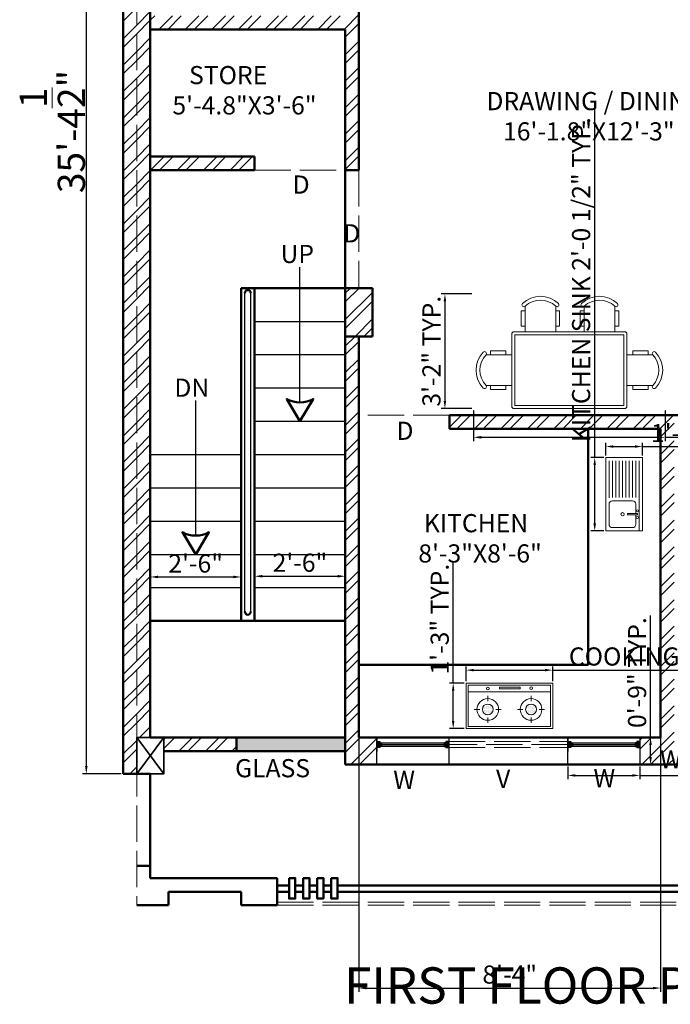
# Model space of a CAD drawing. Units: millimetres. Extents: x 4237 to 5109, y 21391 to 22486.
# Tile 13 of 17: x 4678 to 4894, y 21940 to 22265. Entities that reach past the tile are written whole.
import ezdxf

# ---------------------------------------------------------------- set-up
doc = ezdxf.new("R2010")
doc.units = ezdxf.units.MM
doc.linetypes.add('ACAD_ISO02W100', pattern=[15, 12, -3])
for name, color, linetype, lineweight in [('A-ANNO-DIMS', 2, 'Continuous', 18), ('A-ANNO-TEXT', 7, 'Continuous', 18), ('A-AREA-IDEN', 3, 'Continuous', 18), ('A-FLOR-OVHD', 1, 'ACAD_ISO02W100', 18), ('A-FLOR-STRS', 7, 'Continuous', 25), ('A-FURN', 8, 'Continuous', 18), ('A-WALL', 7, 'Continuous', 50), ('A-WALL-PATT', 252, 'Continuous', 13), ('column', 102, 'Continuous', 35), ('windows', 140, 'Continuous', 25)]:
    doc.layers.add(name, color=color, linetype=linetype, lineweight=lineweight)
doc.styles.get("Standard").update_dxf_attribs({"font": 'arial.ttf'})
doc.dimstyles.new('ISO-25', dxfattribs={"dimtxt": 6, "dimasz": 2.5, "dimexe": 1.25, "dimexo": 0.625, "dimtad": 1, "dimdec": 1, "dimlunit": 4, "dimtxsty": 'Standard', "dimcen": 2.5, "dimadec": 0, "dimazin": 0, "dimtfac": 1, "dimtdec": 1, "dimtmove": 0, "dimatfit": 3, "dimfxl": 1, "dimarcsym": 0})

# ---------------------------------------------------------------- blocks, each defined once
blk = doc.blocks.new('table dinning')
for p, q in [((4388.77, 22272.2), (4387.5, 22272.2)), ((4387.5, 22267.12), (4387.5, 22272.2)), ((4388.77, 22273.66), (4388.77, 22265.14)), ((4398.93, 22265.14), (4398.93, 22273.66)), ((4398.93, 22272.2), (4400.2, 22272.2)), ((4400.2, 22267.12), (4400.2, 22272.2)), ((4388.77, 22267.12), (4387.5, 22267.12)), ((4398.93, 22267.12), (4400.2, 22267.12)), ((4374.21, 22261.13), (4374.21, 22262.4)), ((4379.29, 22262.4), (4374.21, 22262.4)), ((4379.29, 22261.13), (4379.29, 22262.4)), ((4372.74, 22261.13), (4381.15, 22261.13)), ((4381.15, 22250.97), (4372.74, 22250.97)), ((4374.21, 22250.97), (4374.21, 22249.7)), ((4379.29, 22249.7), (4374.21, 22249.7)), ((4379.29, 22250.97), (4379.29, 22249.7)), ((4374.21, 22241.61), (4374.21, 22242.88)), ((4379.29, 22242.88), (4374.21, 22242.88)), ((4379.29, 22241.61), (4379.29, 22242.88)), ((4372.74, 22241.61), (4381.15, 22241.61)), ((4381.15, 22231.45), (4372.74, 22231.45)), ((4374.21, 22231.45), (4374.21, 22230.18)), ((4379.29, 22230.18), (4374.21, 22230.18)), ((4379.29, 22231.45), (4379.29, 22230.18)), ((4388.77, 22218.52), (4388.77, 22227.04)), ((4398.93, 22227.04), (4398.93, 22218.52)), ((4387.5, 22225.06), (4387.5, 22219.98)), ((4388.77, 22225.06), (4387.5, 22225.06)), ((4398.93, 22225.06), (4400.2, 22225.06)), ((4400.2, 22225.06), (4400.2, 22219.98)), ((4388.77, 22219.98), (4387.5, 22219.98)), ((4398.93, 22219.98), (4400.2, 22219.98))]:
    blk.add_line(p, q)
blk.add_lwpolyline([(4381.91, 22265.14), (4405.79, 22265.14, -0.414214), (4406.55, 22264.38), (4406.55, 22227.8, -0.414214), (4405.79, 22227.04), (4381.91, 22227.04, -0.414214), (4381.15, 22227.8), (4381.15, 22264.38, -0.414214)], format="xyb", close=True)
blk.add_lwpolyline([(4382.15, 22264.14), (4405.55, 22264.14), (4405.55, 22228.04), (4382.15, 22228.04)], close=True)
for centre, radius, start, end in [((4393.85, 22268.32), 8.64, 46.4394, 133.5606), ((4393.85, 22268.32), 7.37, 46.4394, 133.5606), ((4388.37, 22274.16), 0.637, 138.3417, 308.7795), ((4399.33, 22274.16), 0.637, 231.2205, 41.6583), ((4372.25, 22261.53), 0.637, 321.2205, 131.6583), ((4378.09, 22256.05), 8.64, 136.4394, 223.5606), ((4378.09, 22256.05), 7.37, 136.4394, 223.5606), ((4372.25, 22250.57), 0.637, 228.3417, 38.7795), ((4372.25, 22242.01), 0.637, 321.2205, 131.6583), ((4378.09, 22236.53), 8.64, 136.4394, 223.5606), ((4378.09, 22236.53), 7.37, 136.4394, 223.5606), ((4372.25, 22231.05), 0.637, 228.3417, 38.7795), ((4388.37, 22218.02), 0.637, 51.2205, 221.6583), ((4393.85, 22223.86), 8.64, 226.4394, 313.5606), ((4393.85, 22223.86), 7.37, 226.4394, 313.5606), ((4399.33, 22218.02), 0.637, 318.3417, 128.7795)]:
    blk.add_arc(centre, radius, start, end)
blk = doc.blocks.new('A$C678C741B')
for p, q in [((720, 378), (0, 378)), ((0, 0), (0, 378)), ((702, 360), (18, 360)), ((18, 18), (18, 360)), ((277, 329.9), (277, 344.2)), ((277, 344.2), (448.4, 344.2)), ((448.4, 329.9), (277, 329.9)), ((448.4, 344.2), (448.4, 329.9)), ((702, 18), (702, 360)), ((720, 0), (720, 378)), ((702, 306), (18, 306)), ((180, 226.9), (180, 271.9)), ((540, 226.9), (540, 271.9)), ((138.6, 174.8), (138.6, 174.8)), ((144.2, 186.1), (144.2, 186.1)), ((149.8, 174.8), (149.8, 174.8)), ((155.5, 186.1), (155.5, 186.1)), ((161.1, 197.3), (161.1, 197.3)), ((161.1, 174.8), (161.1, 174.8)), ((166.7, 186.1), (166.7, 186.1)), ((172.3, 197.3), (172.3, 197.3)), ((172.3, 174.8), (172.3, 174.8)), ((178, 186.1), (178, 186.1)), ((183.6, 197.3), (183.6, 197.3)), ((183.6, 174.8), (183.6, 174.8)), ((189.2, 186.1), (189.2, 186.1)), ((194.8, 197.3), (194.8, 197.3)), ((194.8, 174.8), (194.8, 174.8)), ((200.5, 186.1), (200.5, 186.1)), ((206.1, 174.8), (206.1, 174.8)), ((211.7, 186.1), (211.7, 186.1)), ((217.3, 174.8), (217.3, 174.8)), ((498.6, 174.8), (498.6, 174.8)), ((504.2, 186.1), (504.2, 186.1)), ((509.8, 174.8), (509.8, 174.8)), ((515.5, 186.1), (515.5, 186.1)), ((521.1, 197.3), (521.1, 197.3)), ((521.1, 174.8), (521.1, 174.8)), ((526.7, 186.1), (526.7, 186.1)), ((532.3, 197.3), (532.3, 197.3)), ((532.3, 174.8), (532.3, 174.8)), ((538, 186.1), (538, 186.1)), ((543.6, 197.3), (543.6, 197.3)), ((543.6, 174.8), (543.6, 174.8)), ((549.2, 186.1), (549.2, 186.1)), ((554.8, 197.3), (554.8, 197.3)), ((554.8, 174.8), (554.8, 174.8)), ((560.5, 186.1), (560.5, 186.1)), ((566.1, 174.8), (566.1, 174.8)), ((571.7, 186.1), (571.7, 186.1)), ((577.3, 174.8), (577.3, 174.8)), ((112.5, 159.4), (67.5, 159.4)), ((138.6, 152.3), (138.6, 152.3)), ((144.2, 163.6), (144.2, 163.6)), ((144.2, 141.1), (144.2, 141.1)), ((149.8, 152.3), (149.8, 152.3)), ((149.8, 129.8), (149.8, 129.8)), ((155.5, 163.6), (155.5, 163.6)), ((155.5, 141.1), (155.5, 141.1)), ((161.1, 152.3), (161.1, 152.3)), ((161.1, 129.8), (161.1, 129.8)), ((166.7, 163.6), (166.7, 163.6)), ((166.7, 141.1), (166.7, 141.1)), ((166.7, 118.6), (166.7, 118.6)), ((172.3, 152.3), (172.3, 152.3)), ((172.3, 129.8), (172.3, 129.8)), ((178, 163.6), (178, 163.6)), ((178, 141.1), (178, 141.1)), ((178, 118.6), (178, 118.6)), ((180, 46.9), (180, 91.9)), ((183.6, 152.3), (183.6, 152.3)), ((183.6, 129.8), (183.6, 129.8)), ((189.2, 163.6), (189.2, 163.6)), ((189.2, 141.1), (189.2, 141.1)), ((189.2, 118.6), (189.2, 118.6)), ((194.8, 152.3), (194.8, 152.3)), ((194.8, 129.8), (194.8, 129.8)), ((200.5, 163.6), (200.5, 163.6)), ((200.5, 141.1), (200.5, 141.1)), ((206.1, 152.3), (206.1, 152.3)), ((206.1, 129.8), (206.1, 129.8)), ((211.7, 163.6), (211.7, 163.6)), ((211.7, 141.1), (211.7, 141.1)), ((217.3, 152.3), (217.3, 152.3)), ((223, 163.6), (223, 163.6)), ((292.5, 159.4), (247.5, 159.4)), ((472.5, 159.4), (427.5, 159.4)), ((498.6, 152.3), (498.6, 152.3)), ((504.2, 163.6), (504.2, 163.6)), ((504.2, 141.1), (504.2, 141.1)), ((509.8, 152.3), (509.8, 152.3)), ((509.8, 129.8), (509.8, 129.8)), ((515.5, 163.6), (515.5, 163.6)), ((515.5, 141.1), (515.5, 141.1)), ((521.1, 152.3), (521.1, 152.3)), ((521.1, 129.8), (521.1, 129.8)), ((526.7, 163.6), (526.7, 163.6)), ((526.7, 141.1), (526.7, 141.1)), ((526.7, 118.6), (526.7, 118.6)), ((532.3, 152.3), (532.3, 152.3)), ((532.3, 129.8), (532.3, 129.8)), ((538, 163.6), (538, 163.6)), ((538, 141.1), (538, 141.1)), ((538, 118.6), (538, 118.6)), ((540, 46.9), (540, 91.9)), ((543.6, 152.3), (543.6, 152.3)), ((543.6, 129.8), (543.6, 129.8)), ((549.2, 163.6), (549.2, 163.6)), ((549.2, 141.1), (549.2, 141.1)), ((549.2, 118.6), (549.2, 118.6)), ((554.8, 152.3), (554.8, 152.3)), ((554.8, 129.8), (554.8, 129.8)), ((560.5, 163.6), (560.5, 163.6)), ((560.5, 141.1), (560.5, 141.1)), ((566.1, 152.3), (566.1, 152.3)), ((566.1, 129.8), (566.1, 129.8)), ((571.7, 163.6), (571.7, 163.6)), ((571.7, 141.1), (571.7, 141.1)), ((577.3, 152.3), (577.3, 152.3)), ((583, 163.6), (583, 163.6)), ((652.5, 159.4), (607.5, 159.4)), ((720, 0), (0, 0)), ((702, 18), (18, 18))]:
    blk.add_line(p, q)
for centre, radius in [((180.2, 333.1), 10.8), ((540.5, 336.3), 10.8), ((180, 159.4), 90), ((540, 159.4), 90), ((180, 159.4), 45), ((540, 159.4), 45)]:
    blk.add_circle(centre, radius)
blk = doc.blocks.new('A$C634174F9')
for p, q in [((0, 0), (0, 550)), ((0, 550), (1100, 550)), ((0, 500), (1052, 500)), ((100, 450), (240, 450)), ((241, 479), (241, 328)), ((261, 479), (241, 479)), ((261, 479), (261, 328)), ((261, 450), (400, 450)), ((501, 450), (1052, 450)), ((1100, 550), (1100, 0)), ((50, 100), (50, 400)), ((241, 328), (261, 328)), ((450, 100), (450, 400)), ((501, 400), (1052, 400)), ((501, 350), (1052, 350)), ((501, 300), (1052, 300)), ((501, 250), (1052, 250)), ((501, 200), (1052, 200)), ((501, 150), (1052, 150)), ((1100, 0), (0, 0)), ((400, 50), (100, 50)), ((1052, 50), (498, 50)), ((501, 100), (1052, 100))]:
    blk.add_line(p, q)
for centre, radius in [((201, 474), 15.3), ((301, 474), 15.3), ((251, 254), 25)]:
    blk.add_circle(centre, radius)
for centre, start, end in [((100, 400), 90, 180), ((100, 400), 90, 180), ((400, 400), 0, 90), ((400, 400), 0, 90), ((100, 100), 180, 270), ((400, 100), 270, 0)]:
    blk.add_arc(centre, 50, start, end)
blk = doc.blocks.new('*D52')
at = {"layer": 'A-ANNO-DIMS', "color": 0, "lineweight": -2, "transparency": 16777216}
for p, q in [((4721.61, 22094.28), (4721.61, 22079.97)), ((4751.61, 22094.28), (4751.61, 22079.97)), ((4724.11, 22081.22), (4749.11, 22081.22))]:
    blk.add_line(p, q, dxfattribs=at)
at = {"layer": 'A-ANNO-DIMS', "color": 0, "transparency": 16777216}
for points in [[(4724.11, 22081.64), (4724.11, 22080.81), (4721.61, 22081.22)], [(4749.11, 22081.64), (4749.11, 22080.81), (4751.61, 22081.22)]]:
    blk.add_solid(points, dxfattribs=at)
at = {"layer": 'Defpoints', "color": 0, "transparency": 16777216}
for p in [(4721.61, 22094.9), (4751.61, 22094.9), (4751.61, 22081.22)]:
    blk.add_point(p, dxfattribs=at)
at = {"layer": 'A-ANNO-DIMS', "color": 0, "transparency": 16777216, "insert": (4736.61, 22084.91), "char_height": 6, "attachment_point": 5}
blk.add_mtext('2\'-6"', dxfattribs=at)
blk = doc.blocks.new('*D53')
at = {"layer": 'A-ANNO-DIMS', "color": 0, "lineweight": -2, "transparency": 16777216}
for p, q in [((4756.11, 22081.85), (4756.11, 22082.71)), ((4758.61, 22081.46), (4783.61, 22081.46)), ((4786.11, 22081.85), (4786.11, 22082.71))]:
    blk.add_line(p, q, dxfattribs=at)
at = {"layer": 'A-ANNO-DIMS', "color": 0, "transparency": 16777216}
for points in [[(4758.61, 22081.88), (4758.61, 22081.04), (4756.11, 22081.46)], [(4783.61, 22081.88), (4783.61, 22081.04), (4786.11, 22081.46)]]:
    blk.add_solid(points, dxfattribs=at)
at = {"layer": 'Defpoints', "color": 0, "transparency": 16777216}
for p in [(4756.11, 22081.22), (4786.11, 22081.46), (4786.11, 22081.22)]:
    blk.add_point(p, dxfattribs=at)
at = {"layer": 'A-ANNO-DIMS', "color": 0, "transparency": 16777216, "insert": (4771.11, 22085.15), "char_height": 6, "attachment_point": 5}
blk.add_mtext('2\'-6"', dxfattribs=at)
blk = doc.blocks.new('*D60')
at = {"layer": 'A-ANNO-DIMS', "color": 0, "lineweight": -2, "transparency": 16777216}
for p, q in [((4711.99, 22440.7), (4699.18, 22440.7)), ((4700.43, 22438.2), (4700.43, 22018.7)), ((4711.99, 22016.2), (4699.18, 22016.2))]:
    blk.add_line(p, q, dxfattribs=at)
at = {"layer": 'A-ANNO-DIMS', "color": 0, "transparency": 16777216}
for points in [[(4700.01, 22438.2), (4700.85, 22438.2), (4700.43, 22440.7)], [(4700.01, 22018.7), (4700.85, 22018.7), (4700.43, 22016.2)]]:
    blk.add_solid(points, dxfattribs=at)
at = {"layer": 'Defpoints', "color": 0, "transparency": 16777216}
for p in [(4712.61, 22440.7), (4700.43, 22016.2), (4712.61, 22016.2)]:
    blk.add_point(p, dxfattribs=at)
at = {"layer": 'A-ANNO-DIMS', "color": 0, "transparency": 16777216, "insert": (4689.19, 22228.45), "char_height": 9, "attachment_point": 5, "rotation": 90}
blk.add_mtext('35\'-4{\\H1x;\\S1/2;}"', dxfattribs=at)
blk = doc.blocks.new('WIN-B')
blk.add_line((0, 8.86), (0, 4.36))
blk.add_lwpolyline([(0, 9), (23.8, 9), (23.8, 0), (0, 0)], close=True)
blk = doc.blocks.new('*D82')
at = {"layer": 'A-ANNO-DIMS', "color": 0, "lineweight": -2, "transparency": 16777216}
for p, q in [((4859.72, 22018.58), (4859.72, 22014.38)), ((4883.52, 22018.58), (4883.52, 22014.38)), ((4862.22, 22015.63), (4881.02, 22015.63)), ((4883.52, 22015.63), (5018.13, 22015.63))]:
    blk.add_line(p, q, dxfattribs=at)
at = {"layer": 'A-ANNO-DIMS', "color": 0, "transparency": 16777216}
for points in [[(4862.22, 22016.05), (4862.22, 22015.21), (4859.72, 22015.63)], [(4881.02, 22016.05), (4881.02, 22015.21), (4883.52, 22015.63)]]:
    blk.add_solid(points, dxfattribs=at)
at = {"layer": 'Defpoints', "color": 0, "transparency": 16777216}
for p in [(4859.72, 22019.2), (4883.52, 22019.2), (4883.52, 22015.63)]:
    blk.add_point(p, dxfattribs=at)
at = {"layer": 'A-ANNO-DIMS', "color": 0, "transparency": 16777216, "insert": (4952.07, 22020.19), "char_height": 6, "attachment_point": 5}
blk.add_mtext('WINDOW W (KITCHEN) 2\'-0" TYP.', dxfattribs=at)
blk = doc.blocks.new('*D83')
at = {"layer": 'A-ANNO-DIMS', "color": 0, "lineweight": -2, "transparency": 16777216}
for p, q in [((4887.09, 22028.2), (4887.09, 22068.52)), ((4884.14, 22028.2), (4888.34, 22028.2)), ((4887.09, 22021.7), (4887.09, 22025.7)), ((4884.14, 22019.2), (4888.34, 22019.2))]:
    blk.add_line(p, q, dxfattribs=at)
at = {"layer": 'A-ANNO-DIMS', "color": 0, "transparency": 16777216}
for points in [[(4886.67, 22025.7), (4887.5, 22025.7), (4887.09, 22028.2)], [(4886.67, 22021.7), (4887.5, 22021.7), (4887.09, 22019.2)]]:
    blk.add_solid(points, dxfattribs=at)
at = {"layer": 'Defpoints', "color": 0, "transparency": 16777216}
for p in [(4883.52, 22028.2), (4887.09, 22028.2), (4883.52, 22019.2)]:
    blk.add_point(p, dxfattribs=at)
at = {"layer": 'A-ANNO-DIMS', "color": 0, "transparency": 16777216, "insert": (4883.4, 22049.61), "char_height": 6, "attachment_point": 5, "rotation": 90}
blk.add_mtext('0\'-9" TYP.', dxfattribs=at)
blk = doc.blocks.new('*D86')
at = {"layer": 'A-ANNO-DIMS', "color": 0, "lineweight": -2, "transparency": 16777216}
for p, q in [((4826.09, 22046.76), (4826.09, 22051.68)), ((4854.72, 22046.76), (4854.72, 22051.68)), ((4828.59, 22050.43), (4852.22, 22050.43)), ((4854.72, 22050.43), (4971.36, 22050.43))]:
    blk.add_line(p, q, dxfattribs=at)
at = {"layer": 'A-ANNO-DIMS', "color": 0, "transparency": 16777216}
for points in [[(4828.59, 22050.85), (4828.59, 22050.02), (4826.09, 22050.43)], [(4852.22, 22050.85), (4852.22, 22050.02), (4854.72, 22050.43)]]:
    blk.add_solid(points, dxfattribs=at)
at = {"layer": 'Defpoints', "color": 0, "transparency": 16777216}
for p in [(4854.72, 22050.43), (4826.09, 22046.14), (4854.72, 22046.14)]:
    blk.add_point(p, dxfattribs=at)
at = {"layer": 'A-ANNO-DIMS', "color": 0, "transparency": 16777216, "insert": (4914.29, 22054.16), "char_height": 6, "attachment_point": 5}
blk.add_mtext('COOKING HOB 2\'-4 1/2" TYP.', dxfattribs=at)
blk = doc.blocks.new('*D87')
at = {"layer": 'A-ANNO-DIMS', "color": 0, "lineweight": -2, "transparency": 16777216}
for p, q in [((4821.8, 22046.14), (4821.8, 22085.9)), ((4825.47, 22046.14), (4820.55, 22046.14)), ((4821.8, 22033.61), (4821.8, 22043.64)), ((4825.47, 22031.11), (4820.55, 22031.11))]:
    blk.add_line(p, q, dxfattribs=at)
at = {"layer": 'A-ANNO-DIMS', "color": 0, "transparency": 16777216}
for points in [[(4821.38, 22043.64), (4822.22, 22043.64), (4821.8, 22046.14)], [(4821.38, 22033.61), (4822.22, 22033.61), (4821.8, 22031.11)]]:
    blk.add_solid(points, dxfattribs=at)
at = {"layer": 'Defpoints', "color": 0, "transparency": 16777216}
for p in [(4821.8, 22046.14), (4826.09, 22046.14), (4826.09, 22031.11)]:
    blk.add_point(p, dxfattribs=at)
at = {"layer": 'A-ANNO-DIMS', "color": 0, "transparency": 16777216, "insert": (4818.11, 22067.27), "char_height": 6, "attachment_point": 5, "rotation": 90}
blk.add_mtext('1\'-3" TYP.', dxfattribs=at)
blk = doc.blocks.new('*D88')
at = {"layer": 'A-ANNO-DIMS', "color": 0, "lineweight": -2, "transparency": 16777216}
for p, q in [((4868.61, 22120.69), (4868.61, 22235.74)), ((4871.63, 22120.69), (4867.36, 22120.69)), ((4868.61, 22098.92), (4868.61, 22118.19)), ((4871.63, 22096.42), (4867.36, 22096.42))]:
    blk.add_line(p, q, dxfattribs=at)
at = {"layer": 'A-ANNO-DIMS', "color": 0, "transparency": 16777216}
for points in [[(4868.2, 22118.19), (4869.03, 22118.19), (4868.61, 22120.69)], [(4868.2, 22098.92), (4869.03, 22098.92), (4868.61, 22096.42)]]:
    blk.add_solid(points, dxfattribs=at)
at = {"layer": 'Defpoints', "color": 0, "transparency": 16777216}
for p in [(4868.61, 22120.69), (4872.25, 22120.69), (4872.25, 22096.42)]:
    blk.add_point(p, dxfattribs=at)
at = {"layer": 'A-ANNO-DIMS', "color": 0, "transparency": 16777216, "insert": (4864.89, 22179.47), "char_height": 6, "attachment_point": 5, "rotation": 90}
blk.add_mtext('KITCHEN SINK 2\'-0 1/2" TYP.', dxfattribs=at)
blk = doc.blocks.new('*D89')
at = {"layer": 'A-ANNO-DIMS', "color": 0, "lineweight": -2, "transparency": 16777216}
for p, q in [((4872.25, 22121.32), (4872.25, 22125.58)), ((4884.39, 22121.32), (4884.39, 22125.58)), ((4874.75, 22124.33), (4881.89, 22124.33)), ((4884.39, 22124.33), (4924.15, 22124.33))]:
    blk.add_line(p, q, dxfattribs=at)
at = {"layer": 'A-ANNO-DIMS', "color": 0, "transparency": 16777216}
for points in [[(4874.75, 22124.75), (4874.75, 22123.92), (4872.25, 22124.33)], [(4881.89, 22124.75), (4881.89, 22123.92), (4884.39, 22124.33)]]:
    blk.add_solid(points, dxfattribs=at)
at = {"layer": 'Defpoints', "color": 0, "transparency": 16777216}
for p in [(4884.39, 22124.33), (4872.25, 22120.69), (4884.39, 22120.69)]:
    blk.add_point(p, dxfattribs=at)
at = {"layer": 'A-ANNO-DIMS', "color": 0, "transparency": 16777216, "insert": (4905.52, 22128.02), "char_height": 6, "attachment_point": 5}
blk.add_mtext('1\'-0" TYP.', dxfattribs=at)
blk = doc.blocks.new('*D92')
at = {"layer": 'A-ANNO-DIMS', "color": 0, "lineweight": -2, "transparency": 16777216}
for p, q in [((4828.57, 22136.25), (4828.57, 22126.13)), ((4891.89, 22136.25), (4891.89, 22126.13)), ((4831.07, 22127.38), (4889.39, 22127.38)), ((4891.89, 22127.38), (4996.19, 22127.38))]:
    blk.add_line(p, q, dxfattribs=at)
at = {"layer": 'A-ANNO-DIMS', "color": 0, "transparency": 16777216}
for points in [[(4831.07, 22127.8), (4831.07, 22126.96), (4828.57, 22127.38)], [(4889.39, 22127.8), (4889.39, 22126.96), (4891.89, 22127.38)]]:
    blk.add_solid(points, dxfattribs=at)
at = {"layer": 'Defpoints', "color": 0, "transparency": 16777216}
for p in [(4828.57, 22136.88), (4891.89, 22136.88), (4891.89, 22127.38)]:
    blk.add_point(p, dxfattribs=at)
at = {"layer": 'A-ANNO-DIMS', "color": 0, "transparency": 16777216, "insert": (4945.29, 22131.11), "char_height": 6, "attachment_point": 5}
blk.add_mtext('DINING SET 5\'-3 1/2" TYP.', dxfattribs=at)
blk = doc.blocks.new('*D93')
at = {"layer": 'A-ANNO-DIMS', "color": 0, "lineweight": -2, "transparency": 16777216}
for p, q in [((4827.94, 22174.78), (4817.82, 22174.78)), ((4819.07, 22172.28), (4819.07, 22139.38)), ((4827.94, 22136.88), (4817.82, 22136.88))]:
    blk.add_line(p, q, dxfattribs=at)
at = {"layer": 'A-ANNO-DIMS', "color": 0, "transparency": 16777216}
for points in [[(4818.65, 22172.28), (4819.48, 22172.28), (4819.07, 22174.78)], [(4818.65, 22139.38), (4819.48, 22139.38), (4819.07, 22136.88)]]:
    blk.add_solid(points, dxfattribs=at)
at = {"layer": 'Defpoints', "color": 0, "transparency": 16777216}
for p in [(4828.57, 22174.78), (4819.07, 22136.88), (4828.57, 22136.88)]:
    blk.add_point(p, dxfattribs=at)
at = {"layer": 'A-ANNO-DIMS', "color": 0, "transparency": 16777216, "insert": (4815.38, 22155.83), "char_height": 6, "attachment_point": 5, "rotation": 90}
blk.add_mtext('3\'-2" TYP.', dxfattribs=at)
blk = doc.blocks.new('*D120')
at = {"layer": 'A-ANNO-DIMS', "color": 0, "lineweight": -2, "transparency": 16777216}
for p, q in [((4790.61, 22134.08), (4790.61, 21944.1)), ((4890.41, 22129.58), (4890.41, 21944.1)), ((4793.11, 21945.35), (4887.91, 21945.35))]:
    blk.add_line(p, q, dxfattribs=at)
at = {"layer": 'A-ANNO-DIMS', "color": 0, "transparency": 16777216}
for points in [[(4793.11, 21945.77), (4793.11, 21944.93), (4790.61, 21945.35)], [(4887.91, 21945.77), (4887.91, 21944.93), (4890.41, 21945.35)]]:
    blk.add_solid(points, dxfattribs=at)
at = {"layer": 'Defpoints', "color": 0, "transparency": 16777216}
for p in [(4790.61, 22134.7), (4890.41, 22130.2), (4890.41, 21945.35)]:
    blk.add_point(p, dxfattribs=at)
at = {"layer": 'A-ANNO-DIMS', "color": 0, "transparency": 16777216, "insert": (4840.51, 21949.04), "char_height": 6, "attachment_point": 5}
blk.add_mtext('8\'-4"', dxfattribs=at)

msp = doc.modelspace()

# ---------------------------------------------------------------- hatches: boundary and pattern name
at = {"layer": 'A-WALL-PATT'}
h = msp.add_hatch(dxfattribs=at)
h.set_pattern_fill('ANSI32', color=256, scale=0.65)
h.paths.add_polyline_path([(4717.11, 22440.7), (4712.61, 22440.7), (4712.61, 22016.2), (4717.11, 22016.2), (4717.11, 22028.2)])
h = msp.add_hatch(dxfattribs=at)
h.set_pattern_fill('ANSI32', color=256, scale=0.65)
h.paths.add_polyline_path([(4721.61, 22440.7), (4717.11, 22440.7), (4717.11, 22028.2), (4721.61, 22028.2)])
h = msp.add_hatch(dxfattribs=at)
h.set_pattern_fill('ANSI32', color=256, scale=0.65)
h.paths.add_polyline_path([(4790.61, 22287.7), (4786.11, 22287.7), (4786.11, 22266.7), (4721.61, 22266.7), (4721.61, 22262.2), (4786.11, 22262.2), (4786.11, 22215.7), (4790.61, 22215.7)])
h = msp.add_hatch(dxfattribs=at)
h.set_pattern_fill('ANSI32', color=256, scale=0.65)
h.paths.add_polyline_path([(4756.11, 22220.2), (4721.61, 22220.2), (4721.61, 22215.7), (4756.11, 22215.7)], flags=17)
h = msp.add_hatch(dxfattribs=at)
h.set_pattern_fill('ANSI32', color=256, scale=0.65)
h.paths.add_polyline_path([(4795.11, 22176.7), (4786.11, 22176.7), (4786.11, 22160.75), (4790.61, 22160.75), (4795.11, 22160.75)])
h = msp.add_hatch(dxfattribs=at)
h.set_pattern_fill('ANSI32', color=256, scale=0.65)
h.paths.add_polyline_path([(4796.55, 22028.2), (4790.61, 22028.2), (4790.61, 22160.75), (4786.11, 22160.75), (4786.11, 22019.2), (4796.55, 22019.2)])
h = msp.add_hatch(dxfattribs=at)
h.set_pattern_fill('ANSI32', color=256, scale=0.65)
h.paths.add_polyline_path([(4894.91, 22134.7), (4820.61, 22134.7), (4820.61, 22130.2), (4890.41, 22130.2), (4890.41, 22028.2), (4883.52, 22028.2), (4883.52, 22019.2), (4894.91, 22019.2)])
h = msp.add_hatch(dxfattribs=at)
h.set_pattern_fill('ANSI32', color=256, scale=0.65)
h.paths.add_polyline_path([(4750.11, 22028.2), (4726.11, 22028.2), (4726.11, 22023.7), (4750.11, 22023.7)])
h = msp.add_hatch(color=256, dxfattribs=at)
h.dxf.hatch_style = 1
h.paths.add_polyline_path([(4786.11, 22028.2), (4750.11, 22028.2), (4750.11, 22023.7), (4786.11, 22023.7)])
h = msp.add_hatch(color=256, dxfattribs=at)
h.dxf.hatch_style = 1
h.paths.add_polyline_path([(4798.07, 22026.42), (4797.55, 22026.42), (4797.55, 22026.81), (4796.55, 22026.81), (4796.55, 22024.81), (4797.55, 22024.81), (4797.55, 22025.2), (4798.07, 22025.2)])
h = msp.add_hatch(color=256, dxfattribs=at)
h.dxf.hatch_style = 1
h.paths.add_polyline_path([(4820.35, 22026.81), (4819.35, 22026.81), (4819.35, 22026.42), (4818.84, 22026.42), (4818.84, 22025.2), (4819.35, 22025.2), (4819.35, 22024.81), (4820.35, 22024.81)])
h = msp.add_hatch(color=256, dxfattribs=at)
h.dxf.hatch_style = 1
h.paths.add_polyline_path([(4861.23, 22026.42), (4860.72, 22026.42), (4860.72, 22026.81), (4859.72, 22026.81), (4859.72, 22024.81), (4860.72, 22024.81), (4860.72, 22025.2), (4861.23, 22025.2)])
h = msp.add_hatch(color=256, dxfattribs=at)
h.dxf.hatch_style = 1
h.paths.add_polyline_path([(4883.52, 22026.81), (4882.52, 22026.81), (4882.52, 22026.42), (4882, 22026.42), (4882, 22025.2), (4882.52, 22025.2), (4882.52, 22024.81), (4883.52, 22024.81)])

# ---------------------------------------------------------------- linework, layer by layer
at = {"layer": 'A-FLOR-OVHD'}
for p, q in [((4717.11, 22440.7), (4717.11, 21972.7)), ((4756.11, 22215.7), (4786.11, 22215.7)), ((4790.61, 22215.7), (4790.61, 22176.7)), ((4820.61, 22134.7), (4790.61, 22134.7)), ((4820.35, 22026.81), (4859.72, 22026.81)), ((4859.72, 22025.81), (4820.35, 22025.81)), ((4820.35, 22024.81), (4859.72, 22024.81)), ((4763.61, 21973.7), (5018.1, 21973.7)), ((4763.61, 21972.7), (5020.1, 21972.7))]:
    msp.add_line(p, q, dxfattribs=at)
at = {"layer": 'A-FLOR-STRS'}
for p, q in [((4771.11, 22138.91), (4771.11, 22183.56)), ((4752.86, 22069.76), (4752.86, 22175.06)), ((4754.86, 22069.76), (4754.86, 22175.06)), ((4756.11, 22165.7), (4786.11, 22165.7)), ((4756.11, 22154.7), (4786.11, 22154.7)), ((4756.11, 22143.7), (4786.11, 22143.7)), ((4736.61, 22094.91), (4736.61, 22139.56)), ((4756.11, 22132.7), (4786.11, 22132.7)), ((4721.61, 22121.7), (4751.61, 22121.7)), ((4756.11, 22121.7), (4786.11, 22121.7)), ((4721.61, 22110.7), (4751.61, 22110.7)), ((4756.11, 22110.7), (4786.11, 22110.7)), ((4721.61, 22099.7), (4751.61, 22099.7)), ((4756.11, 22099.7), (4786.11, 22099.7)), ((4721.61, 22088.7), (4751.61, 22088.7)), ((4756.11, 22088.7), (4786.11, 22088.7)), ((4721.61, 22077.7), (4751.61, 22077.7)), ((4756.11, 22077.7), (4786.11, 22077.7))]:
    msp.add_line(p, q, dxfattribs=at)
at = {"layer": 'A-WALL'}
for p, q in [((4712.61, 22440.7), (4712.61, 22016.2)), ((4721.61, 22440.7), (4721.61, 22028.2)), ((4790.61, 22287.7), (4790.61, 22215.7)), ((4721.61, 22262.2), (4786.11, 22262.2)), ((4786.11, 22262.2), (4786.11, 22215.7)), ((4721.61, 22220.2), (4756.11, 22220.2)), ((4756.11, 22220.2), (4756.11, 22215.7)), ((4721.61, 22215.7), (4756.11, 22215.7)), ((4786.11, 22215.7), (4790.61, 22215.7)), ((4786.11, 22215.7), (4786.11, 22176.7)), ((4751.61, 22176.7), (4795.11, 22176.7)), ((4751.61, 22176.7), (4751.61, 22066.7)), ((4756.11, 22176.7), (4756.11, 22066.7)), ((4786.11, 22176.7), (4786.11, 22019.2)), ((4795.11, 22176.7), (4795.11, 22160.75)), ((4786.11, 22160.75), (4795.11, 22160.75)), ((4790.61, 22160.75), (4790.61, 22028.2)), ((4820.61, 22134.7), (4820.61, 22130.2)), ((4820.61, 22134.7), (4899.41, 22134.7)), ((4820.61, 22130.2), (4890.41, 22130.2)), ((4890.41, 22130.2), (4890.41, 22028.2)), ((4721.61, 22066.7), (4786.11, 22066.7)), ((4721.61, 22028.2), (4786.11, 22028.2)), ((4750.11, 22028.2), (4750.11, 22023.7)), ((4790.61, 22028.2), (4890.41, 22028.2)), ((4726.11, 22023.7), (4786.11, 22023.7)), ((4786.11, 22019.2), (4899.41, 22019.2)), ((4721.61, 22016.2), (4712.61, 22016.2)), ((4721.61, 22016.2), (4721.61, 21981.7)), ((4717.11, 21985.7), (4721.61, 21985.7)), ((4721.61, 21981.7), (4763.61, 21981.7)), ((4763.61, 21981.7), (4763.61, 21972.7)), ((4763.61, 21979.2), (4767.5, 21979.2)), ((4769.57, 21979.2), (4772.15, 21979.2)), ((4774.23, 21979.2), (4776.81, 21979.2)), ((4778.89, 21979.2), (4781.47, 21979.2)), ((4783.54, 21979.2), (4901.39, 21979.2)), ((4727.61, 21977.2), (4751.61, 21977.2)), ((4727.61, 21977.2), (4727.61, 21972.7)), ((4751.61, 21977.2), (4751.61, 21972.7)), ((4763.61, 21977.2), (4767.5, 21977.2)), ((4769.57, 21977.2), (4772.15, 21977.2)), ((4774.23, 21977.2), (4776.81, 21977.2)), ((4778.89, 21977.2), (4781.47, 21977.2)), ((4783.54, 21977.2), (5038.01, 21977.2)), ((4717.11, 21972.7), (4727.61, 21972.7)), ((4763.61, 21972.7), (4751.61, 21972.7))]:
    msp.add_line(p, q, dxfattribs=at)
for points in [[(4771.11, 22132.7), (4775.5, 22139.99, -0.245903), (4766.72, 22139.99)], [(4736.61, 22088.7), (4741, 22095.99, -0.245903), (4732.22, 22095.99)]]:
    msp.add_lwpolyline(points, format="xyb", close=True, dxfattribs=at)
msp.add_lwpolyline([(4790.61, 22052.2), (4866.41, 22052.2), (4866.41, 22130.2)], dxfattribs=at)
for points in [[(4767.5, 21981.7), (4769.57, 21981.7), (4769.57, 21974.94), (4767.5, 21974.94)], [(4772.15, 21981.7), (4774.23, 21981.7), (4774.23, 21974.94), (4772.15, 21974.94)], [(4776.81, 21981.7), (4778.89, 21981.7), (4778.89, 21974.94), (4776.81, 21974.94)], [(4781.47, 21981.7), (4783.54, 21981.7), (4783.54, 21974.94), (4781.47, 21974.94)]]:
    msp.add_lwpolyline(points, close=True, dxfattribs=at)
for centre, start, end in [((4753.86, 22175.06), 0, 180), ((4753.86, 22069.76), 180, 0)]:
    msp.add_arc(centre, 1, start, end, dxfattribs=at)
at = {"layer": 'column'}
for p, q in [((4726.11, 22028.2), (4717.11, 22016.2)), ((4717.11, 22028.2), (4726.11, 22016.2))]:
    msp.add_line(p, q, dxfattribs=at)
msp.add_lwpolyline([(4717.11, 22028.2), (4726.11, 22028.2), (4726.11, 22016.2), (4717.11, 22016.2)], close=True, dxfattribs=at)
at = {"layer": 'windows'}
for p, q in [((4820.35, 22028.06), (4820.35, 22019.2)), ((4883.52, 22028.06), (4883.52, 22019.2)), ((4798.07, 22026.42), (4818.84, 22026.42)), ((4798.07, 22025.81), (4818.84, 22025.81)), ((4818.84, 22025.2), (4798.07, 22025.2)), ((4861.23, 22026.42), (4882, 22026.42)), ((4861.23, 22025.81), (4882, 22025.81)), ((4882, 22025.2), (4861.23, 22025.2))]:
    msp.add_line(p, q, dxfattribs=at)
for points in [[(4796.55, 22026.81), (4797.55, 22026.81), (4797.55, 22026.42), (4798.07, 22026.42), (4798.07, 22025.2), (4797.55, 22025.2), (4797.55, 22024.81), (4796.55, 22024.81)], [(4820.35, 22026.81), (4819.35, 22026.81), (4819.35, 22026.42), (4818.84, 22026.42), (4818.84, 22025.2), (4819.35, 22025.2), (4819.35, 22024.81), (4820.35, 22024.81)], [(4859.72, 22026.81), (4860.72, 22026.81), (4860.72, 22026.42), (4861.23, 22026.42), (4861.23, 22025.2), (4860.72, 22025.2), (4860.72, 22024.81), (4859.72, 22024.81)], [(4883.52, 22026.81), (4882.52, 22026.81), (4882.52, 22026.42), (4882, 22026.42), (4882, 22025.2), (4882.52, 22025.2), (4882.52, 22024.81), (4883.52, 22024.81)]]:
    msp.add_lwpolyline(points, dxfattribs=at)

# ---------------------------------------------------------------- block references
at = {"layer": 'A-FURN', "rotation": 270}
msp.add_blockref('table dinning', (-17385.86, 26543.43), dxfattribs=at)
at = {"layer": 'A-FURN', "xscale": -0.0220671414042477, "yscale": 0.0220671414042477, "zscale": 0.0220671414042477, "rotation": 270}
msp.add_blockref('A$C634174F9', (4872.25, 22096.42), dxfattribs=at)
at = {"layer": 'A-FURN', "xscale": 0.0397613605137319, "yscale": 0.0397613605137319, "zscale": 0.0397613605137319}
msp.add_blockref('A$C678C741B', (4826.09, 22031.11), dxfattribs=at)
at = {"layer": 'windows'}
for p in [(4796.55, 22019.2), (4859.72, 22019.2)]:
    msp.add_blockref('WIN-B', p, dxfattribs=at)

# ---------------------------------------------------------------- texts
at = {"layer": 'A-ANNO-TEXT', "attachment_point": 1}
for s, width, insert, char_height in [('    D', 21.7253, (4761.36, 22213.91), 6), ('    D', 21.7253, (4778.1, 22197.79), 6), ('   UP', 21.7253, (4759.17, 22190.97), 6), ('   DN', 21.7253, (4724.06, 22146.77), 6), ('    D', 21.7253, (4795.69, 22132.53), 6), (' GLASS', 72.5927, (4747.8, 22021.02), 6), ('    W', 21.7253, (4794.64, 22017.17), 6), ('    V', 21.7253, (4828.64, 22017.51), 6), ('    W', 21.7253, (4860.87, 22017.73), 6), ('  FIRST FLOOR PLAN', 222.3103, (4778.34, 21952.2), 12)]:
    msp.add_mtext_dynamic_manual_height_columns(s, width=width, gutter_width=12.5, heights=[0], dxfattribs=dict(at, insert=insert, char_height=char_height))
at = {"layer": 'A-AREA-IDEN', "char_height": 6, "attachment_point": 1}
for s, width, insert in [('     STORE\\P  5\'-4.8"X3\'-6"', 55.7646, (4725.25, 22250.09)), (' DRAWING / DINING  \\P    16\'-1.8"X12\'-3"                ', 94.8365, (4830.95, 22241.5)), ('   KITCHEN\\P  8\'-3"X8\'-6"', 55.7646, (4806.59, 22102))]:
    msp.add_mtext_dynamic_manual_height_columns(s, width=width, gutter_width=12.5, heights=[0], dxfattribs=dict(at, insert=insert))

# ---------------------------------------------------------------- dimensions: what is measured, and where the dimension line sits
at = {"layer": 'A-ANNO-DIMS'}
dim = msp.add_linear_dim(base=(4700.43, 22016.2), p1=(4712.61, 22440.7), p2=(4712.61, 22016.2), angle=90, dimstyle='ISO-25', override={"dimtxt": 9, "dimclrd": 0, "dimclre": 0, "dimclrt": 0}, dxfattribs=at)
dim.commit()
dim.dimension.update_dxf_attribs({"geometry": '*D60', "text_midpoint": (4689.19, 22228.45)})
for base, p1, p2, angle, text, picture, middle in [((4868.61, 22120.69), (4872.25, 22096.42), (4872.25, 22120.69), 90, 'KITCHEN SINK <> TYP.', '*D88', (4864.89, 22179.47)), ((4819.07, 22136.88), (4828.57, 22174.78), (4828.57, 22136.88), 270, '<> TYP.', '*D93', (4815.38, 22155.83)), ((4821.8, 22046.14), (4826.09, 22031.11), (4826.09, 22046.14), 90, '<> TYP.', '*D87', (4818.11, 22067.27)), ((4887.09, 22028.2), (4883.52, 22019.2), (4883.52, 22028.2), 90, '<> TYP.', '*D83', (4883.4, 22049.61))]:
    dim = msp.add_linear_dim(base=base, p1=p1, p2=p2, angle=angle, text=text, dimstyle='ISO-25', override={"dimdec": 1, "dimrnd": 0, "dimzin": 1, "dimlunit": 4, "dimfrac": 2}, dxfattribs=at)
    dim.commit()
    dim.dimension.update_dxf_attribs({"geometry": picture, "text_midpoint": middle})
for base, p1, p2, text, picture, middle in [((4891.89, 22127.38), (4828.57, 22136.88), (4891.89, 22136.88), 'DINING SET <> TYP.', '*D92', (4945.29, 22131.11)), ((4884.39, 22124.33), (4872.25, 22120.69), (4884.39, 22120.69), '<> TYP.', '*D89', (4905.52, 22128.02)), ((4854.72, 22050.43), (4826.09, 22046.14), (4854.72, 22046.14), 'COOKING HOB <> TYP.', '*D86', (4914.29, 22054.16)), ((4883.52, 22015.63), (4859.72, 22019.2), (4883.52, 22019.2), 'WINDOW W (KITCHEN) <> TYP.', '*D82', (4952.07, 22020.19))]:
    dim = msp.add_linear_dim(base=base, p1=p1, p2=p2, text=text, dimstyle='ISO-25', override={"dimdec": 1, "dimrnd": 0, "dimzin": 1, "dimlunit": 4, "dimfrac": 2}, dxfattribs=at)
    dim.commit()
    dim.dimension.update_dxf_attribs({"geometry": picture, "text_midpoint": middle})
for base, p1, p2, override, picture, middle in [((4890.41, 21945.35), (4790.61, 22134.7), (4890.41, 22130.2), {"dimdec": 1, "dimlfac": 1, "dimrnd": 0, "dimzin": 1, "dimdsep": 46, "dimlunit": 4, "dimfrac": 2}, '*D120', (4840.51, 21949.04)), ((4751.61, 22081.22), (4721.61, 22094.9), (4751.61, 22094.9), {"dimclrd": 0, "dimclre": 0, "dimclrt": 0}, '*D52', (4736.61, 22084.91)), ((4786.11, 22081.46), (4756.11, 22081.22), (4786.11, 22081.22), {"dimclrd": 0, "dimclre": 0, "dimclrt": 0}, '*D53', (4771.11, 22085.15))]:
    dim = msp.add_linear_dim(base=base, p1=p1, p2=p2, dimstyle='ISO-25', override=override, dxfattribs=at)
    dim.commit()
    dim.dimension.update_dxf_attribs({"geometry": picture, "text_midpoint": middle})

doc.saveas('drawing.dxf')
